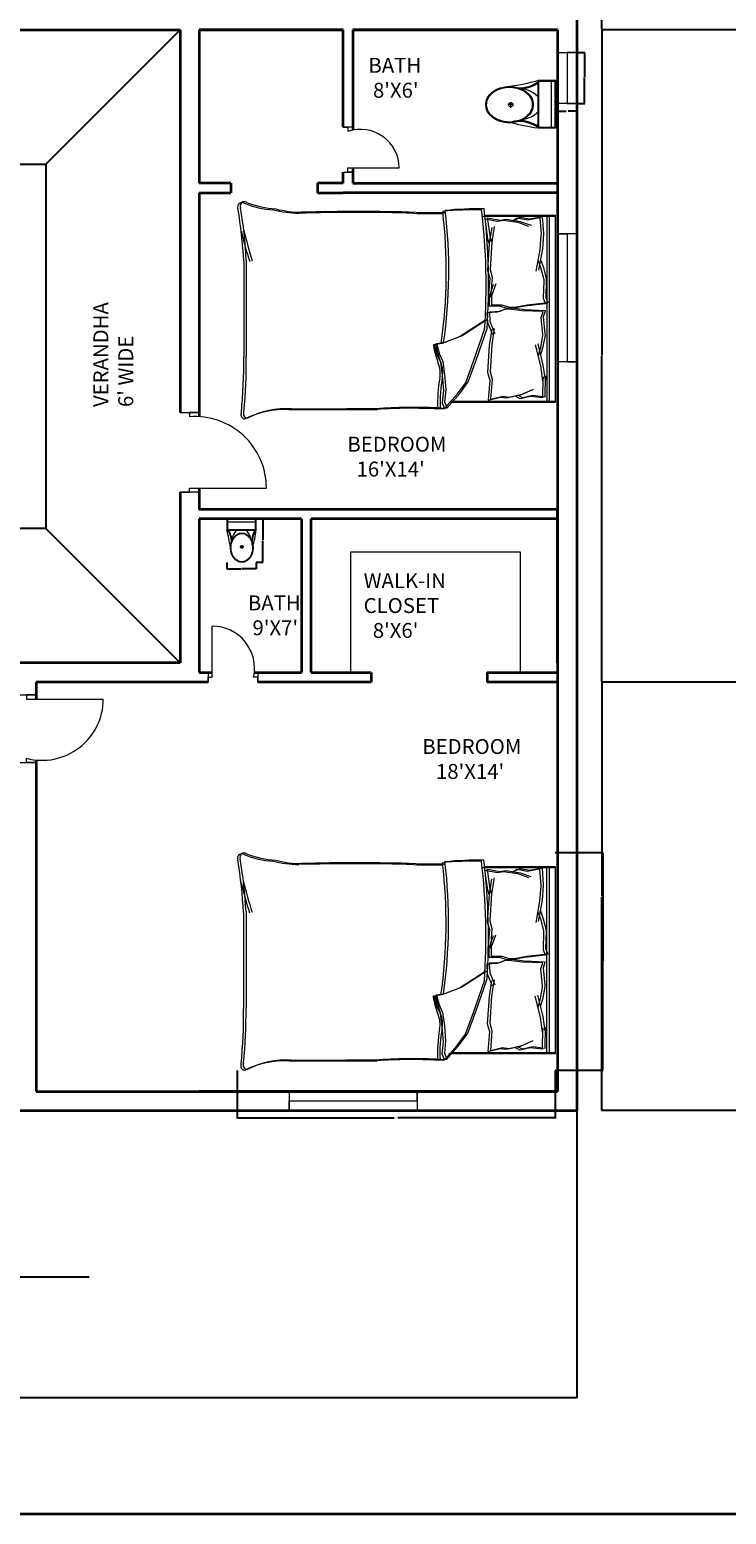
# Model space of a CAD drawing. Units: inches. Extents: x 2185 to 4426, y 1138 to 3073.
# Tile 4 of 14: x 2834 to 3160, y 1138 to 1834. Entities that reach past the tile are written whole.
import ezdxf

# ---------------------------------------------------------------- set-up
doc = ezdxf.new("R2010")
doc.units = ezdxf.units.IN
for name, color, linetype, lineweight in [('A-ANNO-DIMS', 2, 'Continuous', 18), ('A-ANNO-TITL', 7, 'Continuous', 25), ('A-ANNO-TTLB', 7, 'Continuous', 35), ('A-AREA-IDEN', 7, 'Continuous', 18), ('A-DOOR', 3, 'Continuous', 18), ('A-FLOR-CASE', 32, 'Continuous', 18), ('A-FLOR-EDGE', 7, 'Continuous', 25), ('A-FLOR-FIXT', 9, 'Continuous', 18), ('A-FURN', 8, 'Continuous', 18), ('A-GLAZ', 4, 'Continuous', 18), ('A-WALL', 7, 'Continuous', 35)]:
    doc.layers.add(name, color=color, linetype=linetype, lineweight=lineweight)
doc.styles.get("Standard").update_dxf_attribs({"font": 'arial.ttf'})
doc.dimstyles.get("Standard").update_dxf_attribs({"dimtxt": 0.18, "dimasz": 0.18, "dimexe": 0.18, "dimexo": 0.0625, "dimgap": 0.09, "dimtad": 0, "dimtih": 1, "dimtoh": 1, "dimdec": 4, "dimzin": 0, "dimdsep": 46, "dimtxsty": 'Standard', "dimcen": 0.09, "dimadec": 0, "dimazin": 0, "dimtfac": 1, "dimtdec": 4, "dimtofl": 0, "dimtmove": 0, "dimatfit": 3, "dimfxl": 1, "dimtolj": 1, "dimtzin": 0, "dimarcsym": 0})

# ---------------------------------------------------------------- blocks, each defined once
blk = doc.blocks.new('A$C31115884')
for p, q in [((283, 498), (223, 498)), ((258, 466), (258, 523)), ((0, 200), (0, 0)), ((520, 200), (0, 200)), ((10, 190), (10, 10)), ((510, 190), (10, 190)), ((510, 10), (510, 190)), ((520, 0), (520, 200)), ((510, 54), (0, 54)), ((10, 10), (510, 10)), ((0, 0), (520, 0))]:
    blk.add_line(p, q)
blk.add_circle((256, 496), 23.6)
for centre, radius, start, end in [((2778, -205), 2807, 165.4549, 171.7133), ((3237, 905), 2807, 188.2867, 194.5451), ((-295, 403), 365, 324.2091, 9.3499), ((-295, 403), 375, 324.2091, 9.3499), ((384, 406), 293, 190.2774, 224.1564), ((139, 406), 293, 315.8436, 2.6563), ((806, 403), 375, 179.2036, 215.7909), ((806, 403), 365, 170.6501, 215.7909)]:
    blk.add_arc(centre, radius, start, end)
blk.add_ellipse((256, 510), major_axis=(0, -261), ratio=0.772727)
blk.add_open_spline([(256, 259), (263, 259), (270, 260), (288, 262), (299, 265), (320, 273), (330, 278), (350, 291), (360, 299), (378, 316), (386, 326), (402, 347), (409, 358), (421, 383), (427, 395), (436, 422), (440, 436), (445, 465), (447, 480), (448, 509), (448, 524), (445, 553), (443, 568), (436, 596), (432, 610), (422, 636), (416, 649), (402, 672), (395, 683), (379, 703), (370, 712), (351, 728), (341, 735), (321, 746), (310, 751), (289, 757), (278, 759), (256, 761), (245, 761), (223, 757), (212, 754), (191, 746), (181, 741), (161, 728), (151, 720), (133, 703), (125, 693), (110, 672), (103, 660), (90, 636), (85, 623), (76, 596), (72, 582), (67, 553), (66, 538), (64, 509), (65, 494), (68, 465), (70, 450), (77, 422), (81, 408), (91, 382), (97, 370), (111, 346), (118, 335), (135, 316), (144, 307), (162, 291), (172, 284), (193, 273), (203, 269), (225, 262), (236, 260), (250, 259), (253, 259), (256, 259)], degree=3, knots=[0, 0, 0, 0, 0.110105, 0.110105, 0.285049, 0.285049, 0.459994, 0.459994, 0.634938, 0.634938, 0.809882, 0.809882, 0.984827, 0.984827, 1.159771, 1.159771, 1.334715, 1.334715, 1.50966, 1.50966, 1.684604, 1.684604, 1.859549, 1.859549, 2.034493, 2.034493, 2.209437, 2.209437, 2.384382, 2.384382, 2.559326, 2.559326, 2.73427, 2.73427, 2.909215, 2.909215, 3.084159, 3.084159, 3.259103, 3.259103, 3.434048, 3.434048, 3.608992, 3.608992, 3.783936, 3.783936, 3.958881, 3.958881, 4.133825, 4.133825, 4.30877, 4.30877, 4.483714, 4.483714, 4.658658, 4.658658, 4.833603, 4.833603, 5.008547, 5.008547, 5.183491, 5.183491, 5.358436, 5.358436, 5.53338, 5.53338, 5.708324, 5.708324, 5.883269, 5.883269, 6.058213, 6.058213, 6.233158, 6.233158, 6.283185, 6.283185, 6.283185, 6.283185])
blk = doc.blocks.new('BED-DOUBLE')
for p, q in [((0, 93.75), (0, 94.16)), ((0, 94.16), (1.36, 94.16)), ((0, 93.75), (48.66, 93.75)), ((0, 6.35), (0, 93.75)), ((1.17, 94.16), (49.83, 94.16)), ((2.8, 6.35), (2.8, 93.75)), ((3.97, 6.77), (3.97, 94.16)), ((4.68, 91.64), (4.5, 81.76)), ((4.68, 91.64), (10.55, 90.94)), ((5.85, 92.05), (5.67, 82.18)), ((5.85, 92.05), (11.72, 91.36)), ((10.55, 90.94), (15.25, 92.03)), ((16.27, 90.59), (11.37, 88.43)), ((11.72, 91.36), (16.42, 92.45)), ((21.63, 91.64), (15.1, 90.17)), ((15.25, 92.03), (17.16, 91.09)), ((22.8, 92.05), (16.27, 90.59)), ((16.42, 92.45), (18.33, 91.51)), ((24.57, 91.29), (21.63, 91.64)), ((25.74, 91.71), (22.8, 92.05)), ((30.31, 92.71), (24.57, 91.29)), ((31.48, 93.13), (25.74, 91.71)), ((29.57, 83.32), (30.31, 92.71)), ((30.74, 83.74), (31.48, 93.13)), ((50.74, 96.68), (44.79, 89.9)), ((51.91, 97.09), (45.96, 90.32)), ((53.93, 96.82), (50.74, 96.68, 7.08)), ((51.87, 93.87), (50.74, 96.68)), ((51.3, 88.2), (51.87, 93.87)), ((55.1, 97.24), (51.91, 97.09, 7.08)), ((53.04, 94.28), (51.91, 97.09)), ((52.47, 88.62), (53.04, 94.28)), ((4.5, 81.76), (4.65, 83.59)), ((4.65, 83.59), (5.61, 76.65)), ((5.67, 82.18), (5.82, 84.01)), ((5.82, 84.01), (6.78, 77.06)), ((15.1, 90.17), (10.2, 88.01)), ((31.76, 80.16), (30.74, 83.74)), ((40.83, 84.52), (37.15, 74.32)), ((42, 84.94), (38.32, 74.74)), ((44.79, 89.9), (40.83, 84.52)), ((45.96, 90.32), (42, 84.94)), ((51.87, 81.12), (51.3, 88.2)), ((53.04, 81.54), (52.47, 88.62)), ((5.61, 76.65), (8.09, 66.74)), ((6.78, 77.06), (9.26, 67.15)), ((30.59, 79.74), (29.57, 83.32)), ((29.8, 66.92), (30.59, 79.74)), ((30.97, 67.34), (31.76, 80.16)), ((52.72, 74.89), (51.87, 81.12)), ((53.89, 75.31), (53.04, 81.54)), ((6.72, 71.68), (5.63, 67.91)), ((7.89, 72.1), (6.8, 68.32)), ((37.15, 74.32), (31.79, 59.08)), ((38.32, 74.74), (32.96, 59.49)), ((54.42, 71.21), (52.72, 74.89)), ((55.59, 71.63), (53.89, 75.31)), ((55.55, 66.68), (54.42, 71.21)), ((56.72, 67.09), (55.59, 71.63)), ((144.91, 27.55), (144.91, 72.56)), ((146.08, 27.96), (146.08, 72.97)), ((5.63, 67.91), (4.64, 62.55)), ((6.8, 68.32), (5.81, 62.97)), ((5.81, 62.97), (5.85, 62.38)), ((28.58, 59.55), (29.8, 66.92)), ((29.75, 59.97), (30.97, 67.34)), ((31.79, 55.33), (43.66, 63)), ((32.96, 55.75), (44.83, 63.41)), ((43.66, 63), (51.87, 66.11)), ((44.83, 63.41), (53.04, 66.53)), ((51.87, 66.11), (55.55, 66.68)), ((53.04, 66.53), (56.72, 67.09)), ((4.64, 62.55), (4.68, 61.96)), ((4.68, 61.96), (5.45, 53.86)), ((5.85, 62.38), (6.62, 54.28)), ((30.61, 56.23), (28.26, 61.85)), ((31.78, 56.65), (29.43, 62.26)), ((30.89, 51.75), (30.61, 56.23)), ((32.06, 52.16), (31.78, 56.65)), ((5.45, 53.86), (4.56, 51.16)), ((4.56, 51.16), (14.39, 50.71)), ((4.59, 47.93), (14.37, 48.99)), ((6.62, 54.28), (5.73, 51.58)), ((5.73, 51.58), (15.56, 51.13)), ((13.2, 48.57), (19.02, 49.63)), ((14.37, 48.99), (20.19, 50.05)), ((14.39, 50.71), (20.26, 50.02)), ((15.56, 51.13), (21.43, 50.44)), ((19.02, 49.63), (21.4, 49.63)), ((20.19, 50.05), (22.57, 50.05)), ((20.26, 50.02), (22.63, 50.17)), ((21.4, 49.63), (24.84, 48.57)), ((21.43, 50.44), (23.8, 50.59)), ((22.57, 50.05), (26.01, 48.99)), ((22.63, 50.17), (26, 51.44)), ((23.8, 50.59), (27.17, 51.86)), ((26, 51.44), (30.89, 51.75)), ((26.01, 48.99), (30.91, 48.99)), ((27.17, 51.86), (32.06, 52.16)), ((30.91, 48.99), (30.91, 44.49)), ((3.42, 47.51), (13.2, 48.57)), ((4.48, 44.87), (3.42, 47.51)), ((4.21, 36.74), (4.48, 44.87)), ((5.65, 45.29), (4.59, 47.93)), ((5.38, 37.16), (5.65, 45.29)), ((24.84, 48.57), (29.74, 48.57)), ((29.74, 44.08), (27.75, 38.33)), ((30.91, 44.49), (28.91, 38.74)), ((29.57, 35.45), (30.31, 44.83)), ((29.74, 48.57), (29.74, 44.08)), ((30.74, 35.86), (31.48, 45.25)), ((4.21, 36.15), (4.21, 36.74)), ((5.54, 30.86), (4.21, 36.15)), ((5.38, 36.57), (5.38, 37.16)), ((6.7, 31.28), (5.38, 36.57)), ((30.59, 31.86), (29.57, 35.45)), ((31.76, 32.28), (30.74, 35.86)), ((6.86, 27.16), (5.54, 30.86)), ((6.06, 22.14), (7.92, 32.19)), ((8.03, 27.58), (6.7, 31.28)), ((7.23, 22.56), (9.08, 32.6)), ((29.8, 19.04), (30.59, 31.86)), ((30.97, 19.46), (31.76, 32.28)), ((5.54, 15.15), (6.06, 22.14)), ((6.7, 15.57), (7.23, 22.56)), ((5.5, 14.96), (5.54, 15.15)), ((6.1, 7.13), (5.5, 14.96)), ((6.67, 15.37), (6.7, 15.57)), ((7.27, 7.55), (6.67, 15.37)), ((28.58, 11.67), (29.8, 19.04)), ((29.75, 12.09), (30.97, 19.46)), ((29.8, 19.04), (30.39, 16.97)), ((30.39, 16.97), (31.71, 7.65)), ((30.97, 19.46), (31.56, 17.39)), ((31.56, 17.39), (32.88, 8.07)), ((6.06, 7.12), (11.88, 8.18)), ((7.23, 7.54), (13.05, 8.6)), ((16.38, 9.24), (11.35, 11.09)), ((11.88, 8.18), (16.64, 7.39)), ((17.55, 9.65), (12.52, 11.5)), ((13.05, 8.6), (17.81, 7.8)), ((22.99, 8.18), (16.38, 9.24)), ((16.64, 7.39), (18.49, 8.44)), ((24.16, 8.6), (17.55, 9.65)), ((17.81, 7.8), (19.66, 8.86)), ((25.89, 8.71), (22.99, 8.18)), ((27.06, 9.13), (24.16, 8.6)), ((31.71, 7.65), (25.89, 8.71)), ((32.88, 8.07), (27.06, 9.13)), ((1.17, 6.77), (0, 6.77)), ((33.12, 6.35), (0, 6.35)), ((34.29, 6.77), (1.17, 6.77))]:
    blk.add_line(p, q)
for centre, radius, start, end in [((125.19, -8244.52), 8342.06, 90.002168, 90.286887), ((125.57, 139.26), 42.18, 267.47136, 296.46809), ((126.74, 139.68), 42.18, 267.47136, 296.46809), ((144.23, 99.5), 2.02, 332.65876, 86.02002), ((388.18, 75.25), 243.28, 174.4998, 180.63509), ((145.4, 99.91), 2.02, 332.65876, 86.02002), ((389.35, 75.67), 243.28, 174.4998, 180.63509), ((-12.17, 93.86), 66.17, 349.87628, 2.56571), ((66.41, 333.3), 236.81, 266.97912, 273.83645), ((-11, 94.28), 66.17, 349.87628, 2.56571), ((67.58, 333.72), 236.81, 266.97912, 273.83645), ((124.02, -8244.93), 8342.06, 90.002168, 90.286887), ((64.12, 79.99), 11.38, 168.6608, 203.73842), ((65.29, 80.41), 11.38, 168.6608, 203.73842), ((2.71, 56.97), 54.23, 10.66171, 19.88058), ((3.88, 57.39), 54.23, 10.66171, 19.88058), ((285.85, 32.47), 235.93, 171.78449, 186.90062), ((287.02, 32.89), 235.93, 171.78449, 186.90062), ((55.66, 66.99), 0.337, 250.24637, 1.13765), ((56.83, 67.41), 0.337, 250.24637, 1.13765), ((332.91, 39.06), 301.67, 176.08655, 186.78213), ((334.08, 39.47), 301.67, 176.08655, 186.78213), ((-42.19, -31.08), 194.68, 13.38322, 17.70533), ((368.43, 39.6), 222.65, 182.99578, 189.40907), ((-43.36, -31.49), 194.68, 13.38322, 17.70533), ((367.26, 39.18), 222.65, 182.99578, 189.40907), ((36.75, 155.73), 152.34, 268.72178, 275.60397), ((37.92, 156.15), 152.34, 268.72178, 275.60397), ((57.01, -305.95), 311.07, 88.4762, 91.00819), ((58.18, -305.53), 311.07, 88.4762, 91.00819), ((92.56, 886.57), 881.98, 268.22771, 271.71854), ((93.72, 886.99), 881.98, 268.22771, 271.71854), ((117.98, -49.19), 54.19, 76.06484, 88.91125), ((119.15, -48.77), 54.19, 76.06484, 88.91125), ((128.51, -39.61), 43.09, 67.97508, 86.652), ((129.68, -39.19), 43.09, 67.97508, 86.652), ((145.78, 1.99), 1.99, 236.17358, 23.47814), ((146.95, 2.41), 1.99, 236.17358, 23.47814)]:
    blk.add_arc(centre, radius, start, end)
blk = doc.blocks.new('DOOR-SGL-24-BATH-S')
for p, q in [((2, 2.25), (2, 26.25)), ((0, 4.5), (0, 0)), ((0, 0), (0, 2.25)), ((0, 2.25), (0, 2.25)), ((0, 2.25), (2, 2.25)), ((23.36, 2.25), (21.36, 2.25)), ((23.36, 4.5), (23.36, 4.5)), ((23.36, 4.5), (23.36, 0)), ((23.36, 0), (23.36, 2.25))]:
    blk.add_line(p, q)
blk.add_arc((2, 6.44), 19.81, 347.78651, 90)
blk = doc.blocks.new('DOOR-SGL-36-BED-SE')
for p, q in [((0, 37.45), (9, 37.45)), ((9, 37.45), (4.5, 37.45)), ((4.5, 37.45), (4.5, 35.45)), ((9, 0), (0, 0)), ((0, 0), (4.5, 0)), ((4.5, 0), (4.5, 2)), ((4.5, 2), (40.5, 2))]:
    blk.add_line(p, q)
blk.add_arc((6.96, 2), 33.54, 0, 94.21362)
blk = doc.blocks.new('DOOR-SGL-24-BATH-E')
for p, q in [((4.5, 21.05), (0, 21.05)), ((0, 21.05), (2.25, 21.05)), ((2.25, 21.05), (2.25, 19.05)), ((0, 0), (4.5, 0)), ((2.25, 0), (2.25, 2)), ((2.25, 2), (26.25, 2)), ((4.5, 0), (2.25, 0))]:
    blk.add_line(p, q)
blk.add_arc((8.19, 2), 18.06, 0, 109.21567)
blk = doc.blocks.new('DOOR-SGL-36-BED-S')
for p, q in [((0, 31.73), (9, 31.73)), ((9, 31.73), (4.5, 31.73)), ((4.5, 31.73), (4.5, 31.73)), ((4.5, 31.73), (4.5, 29.73)), ((4.5, 29.73), (40.5, 29.73)), ((0, 0), (9, 0)), ((4.5, 0), (4.5, 2)), ((9, 0), (4.5, 0))]:
    blk.add_line(p, q)
blk.add_arc((11.82, 29.73), 28.68, 255.21093, 0)
blk = doc.blocks.new('WIN-PLAN-24IN-03')
for p, q in [((0, 24), (9, 24)), ((9, 24), (4.5, 24)), ((4.5, 24), (4.5, 0)), ((9, 0), (0, 0)), ((4.5, 0), (9, 0))]:
    blk.add_line(p, q)
blk = doc.blocks.new('WIN-PLAN-60IN-01')
for p, q in [((0, 9), (0, 0)), ((60, 4.5), (60, 9)), ((60, 9), (60, 0)), ((0, 0), (0, 4.5)), ((0, 4.5), (0, 4.5)), ((0, 4.5), (60, 4.5))]:
    blk.add_line(p, q)
blk = doc.blocks.new('WARDROBE-U')
for p, q in [((0, 0), (0, 56.6)), ((0, 56.6), (79.32, 56.6)), ((79.32, 56.6), (79.32, 0))]:
    blk.add_line(p, q)
blk = doc.blocks.new('*D46')
at = {"layer": 'A-ANNO-DIMS', "color": 0, "lineweight": -2, "transparency": 16777216}
for p, q in [((2930.76, 1346.2), (2930.76, 1323.71)), ((3079.88, 1346.2), (3079.88, 1323.71)), ((2930.94, 1323.89), (3004.43, 1323.89)), ((3079.7, 1323.89), (3006.21, 1323.89))]:
    blk.add_line(p, q, dxfattribs=at)
at = {"layer": 'A-ANNO-DIMS', "color": 0, "transparency": 16777216}
for points in [[(2930.94, 1323.92), (2930.94, 1323.86), (2930.76, 1323.89)], [(3079.7, 1323.92), (3079.7, 1323.86), (3079.88, 1323.89)]]:
    blk.add_solid(points, dxfattribs=at)
at = {"layer": 'Defpoints', "color": 0, "transparency": 16777216}
for p in [(2930.76, 1346.26), (3079.88, 1346.26), (2930.76, 1323.89)]:
    blk.add_point(p, dxfattribs=at)
at = {"layer": 'A-ANNO-DIMS', "color": 0, "transparency": 16777216, "insert": (3005.32, 1323.89), "char_height": 0.18, "attachment_point": 5}
blk.add_mtext('\\A1;BED 149 TYP.', dxfattribs=at)
blk = doc.blocks.new('*D47')
at = {"layer": 'A-ANNO-DIMS', "color": 0, "lineweight": -2, "transparency": 16777216}
for p, q in [((3079.94, 1448.35), (3102.43, 1448.35)), ((3102.25, 1448.17), (3102.25, 1397.49)), ((3102.25, 1346.44), (3102.25, 1397.12)), ((3079.94, 1346.26), (3102.43, 1346.26))]:
    blk.add_line(p, q, dxfattribs=at)
at = {"layer": 'A-ANNO-DIMS', "color": 0, "transparency": 16777216}
for points in [[(3102.22, 1448.17), (3102.28, 1448.17), (3102.25, 1448.35)], [(3102.22, 1346.44), (3102.28, 1346.44), (3102.25, 1346.26)]]:
    blk.add_solid(points, dxfattribs=at)
at = {"layer": 'Defpoints', "color": 0, "transparency": 16777216}
for p in [(3079.88, 1448.35), (3079.88, 1346.26), (3102.25, 1346.26)]:
    blk.add_point(p, dxfattribs=at)
at = {"layer": 'A-ANNO-DIMS', "color": 0, "transparency": 16777216, "insert": (3102.25, 1397.3), "char_height": 0.18, "attachment_point": 5}
blk.add_mtext('\\A1;102 TYP.', dxfattribs=at)
blk = doc.blocks.new('*D50')
at = {"layer": 'A-ANNO-DIMS', "color": 0, "lineweight": -2, "transparency": 16777216}
for p, q in [((2939.8, 1604.88), (2942.96, 1604.88)), ((2942.78, 1604.7), (2942.78, 1594.9)), ((2942.78, 1584.73), (2942.78, 1594.53)), ((2939.8, 1584.55), (2942.96, 1584.55))]:
    blk.add_line(p, q, dxfattribs=at)
at = {"layer": 'A-ANNO-DIMS', "color": 0, "transparency": 16777216}
for points in [[(2942.75, 1604.7), (2942.81, 1604.7), (2942.78, 1604.88)], [(2942.75, 1584.73), (2942.81, 1584.73), (2942.78, 1584.55)]]:
    blk.add_solid(points, dxfattribs=at)
at = {"layer": 'Defpoints', "color": 0, "transparency": 16777216}
for p in [(2939.73, 1604.88), (2939.73, 1584.55), (2942.78, 1584.55)]:
    blk.add_point(p, dxfattribs=at)
at = {"layer": 'A-ANNO-DIMS', "color": 0, "transparency": 16777216, "insert": (2942.78, 1594.71), "char_height": 0.18, "attachment_point": 5}
blk.add_mtext('\\A1;WC 20', dxfattribs=at)
blk = doc.blocks.new('*D51')
at = {"layer": 'A-ANNO-DIMS', "color": 0, "lineweight": -2, "transparency": 16777216}
for p, q in [((2926.02, 1584.49), (2926.02, 1581.32)), ((2926.2, 1581.5), (2932.66, 1581.5)), ((2939.55, 1581.5), (2933.08, 1581.5)), ((2939.73, 1584.49), (2939.73, 1581.32))]:
    blk.add_line(p, q, dxfattribs=at)
at = {"layer": 'A-ANNO-DIMS', "color": 0, "transparency": 16777216}
for points in [[(2926.2, 1581.53), (2926.2, 1581.47), (2926.02, 1581.5)], [(2939.55, 1581.53), (2939.55, 1581.47), (2939.73, 1581.5)]]:
    blk.add_solid(points, dxfattribs=at)
at = {"layer": 'Defpoints', "color": 0, "transparency": 16777216}
for p in [(2926.02, 1584.55), (2926.02, 1581.5), (2939.73, 1584.55)]:
    blk.add_point(p, dxfattribs=at)
at = {"layer": 'A-ANNO-DIMS', "color": 0, "transparency": 16777216, "insert": (2932.87, 1581.5), "char_height": 0.18, "attachment_point": 5}
blk.add_mtext('\\A1;14', dxfattribs=at)
blk = doc.blocks.new('*D94')
at = {"layer": 'A-ANNO-DIMS', "color": 0, "lineweight": -2, "transparency": 16777216}
for p, q in [((3090.08, 1823.71), (3093.8, 1823.71)), ((3093.62, 1823.53), (3093.62, 1811.9)), ((3093.62, 1799.89), (3093.62, 1811.53)), ((3090.08, 1799.71), (3093.8, 1799.71))]:
    blk.add_line(p, q, dxfattribs=at)
at = {"layer": 'A-ANNO-DIMS', "color": 0, "transparency": 16777216}
for points in [[(3093.59, 1823.53), (3093.65, 1823.53), (3093.62, 1823.71)], [(3093.59, 1799.89), (3093.65, 1799.89), (3093.62, 1799.71)]]:
    blk.add_solid(points, dxfattribs=at)
at = {"layer": 'Defpoints', "color": 0, "transparency": 16777216}
for p in [(3090.02, 1823.71), (3093.62, 1823.71), (3090.02, 1799.71)]:
    blk.add_point(p, dxfattribs=at)
at = {"layer": 'A-ANNO-DIMS', "color": 0, "transparency": 16777216, "insert": (3093.62, 1811.71), "char_height": 0.18, "attachment_point": 5}
blk.add_mtext('\\A1;WINDOW 24 TYP.', dxfattribs=at)
blk = doc.blocks.new('*D95')
at = {"layer": 'A-ANNO-DIMS', "color": 0, "lineweight": -2, "transparency": 16777216}
for p, q in [((3081.02, 1799.65), (3081.02, 1795.93)), ((3090.02, 1799.65), (3090.02, 1795.93)), ((3081.2, 1796.11), (3085.06, 1796.11)), ((3089.84, 1796.11), (3085.98, 1796.11))]:
    blk.add_line(p, q, dxfattribs=at)
at = {"layer": 'A-ANNO-DIMS', "color": 0, "transparency": 16777216}
for points in [[(3081.2, 1796.14), (3081.2, 1796.08), (3081.02, 1796.11)], [(3089.84, 1796.14), (3089.84, 1796.08), (3090.02, 1796.11)]]:
    blk.add_solid(points, dxfattribs=at)
at = {"layer": 'Defpoints', "color": 0, "transparency": 16777216}
for p in [(3081.02, 1799.71), (3090.02, 1799.71), (3090.02, 1796.11)]:
    blk.add_point(p, dxfattribs=at)
at = {"layer": 'A-ANNO-DIMS', "color": 0, "transparency": 16777216, "insert": (3085.52, 1796.11), "char_height": 0.18, "attachment_point": 5}
blk.add_mtext('\\A1;9 TYP.', dxfattribs=at)
blk = doc.blocks.new('*D138')
at = {"layer": 'A-ANNO-DIMS', "color": 0, "lineweight": -2, "transparency": 16777216}
for p, q in [((2368.52, 1327.31), (2368.52, 1192.47)), ((3090.02, 1327.31), (3090.02, 1192.47)), ((2368.7, 1192.65), (2728.88, 1192.65)), ((3089.84, 1192.65), (2729.66, 1192.65))]:
    blk.add_line(p, q, dxfattribs=at)
at = {"layer": 'A-ANNO-DIMS', "color": 0, "transparency": 16777216}
for points in [[(2368.7, 1192.68), (2368.7, 1192.62), (2368.52, 1192.65)], [(3089.84, 1192.68), (3089.84, 1192.62), (3090.02, 1192.65)]]:
    blk.add_solid(points, dxfattribs=at)
at = {"layer": 'Defpoints', "color": 0, "transparency": 16777216}
for p in [(2368.52, 1327.38), (3090.02, 1327.38), (3090.02, 1192.65)]:
    blk.add_point(p, dxfattribs=at)
at = {"layer": 'A-ANNO-DIMS', "color": 0, "transparency": 16777216, "insert": (2729.27, 1192.65), "char_height": 0.18, "attachment_point": 5}
blk.add_mtext('\\A1;721.5', dxfattribs=at)
blk = doc.blocks.new('*D150')
at = {"layer": 'A-ANNO-DIMS', "color": 0, "lineweight": -2, "transparency": 16777216}
for p, q in [((3219.79, 1528.38), (3101.64, 1528.38)), ((3101.82, 1528.2), (3101.82, 1428.06)), ((3101.82, 1327.56), (3101.82, 1427.7)), ((3210.79, 1327.38), (3101.64, 1327.38))]:
    blk.add_line(p, q, dxfattribs=at)
at = {"layer": 'A-ANNO-DIMS', "color": 0, "transparency": 16777216}
for points in [[(3101.79, 1528.2), (3101.85, 1528.2), (3101.82, 1528.38)], [(3101.79, 1327.56), (3101.85, 1327.56), (3101.82, 1327.38)]]:
    blk.add_solid(points, dxfattribs=at)
at = {"layer": 'Defpoints', "color": 0, "transparency": 16777216}
for p in [(3101.82, 1528.38), (3219.85, 1528.38), (3210.85, 1327.38)]:
    blk.add_point(p, dxfattribs=at)
at = {"layer": 'A-ANNO-DIMS', "color": 0, "transparency": 16777216, "insert": (3101.82, 1427.88), "char_height": 0.18, "attachment_point": 5}
blk.add_mtext('\\A1;201', dxfattribs=at)
blk = doc.blocks.new('*D151')
at = {"layer": 'A-ANNO-DIMS', "color": 0, "lineweight": -2, "transparency": 16777216}
for p, q in [((3219.79, 1834.38), (3101.64, 1834.38)), ((3101.82, 1834.2), (3101.82, 1681.56)), ((3101.82, 1528.56), (3101.82, 1681.19)), ((3219.79, 1528.38), (3101.64, 1528.38))]:
    blk.add_line(p, q, dxfattribs=at)
at = {"layer": 'A-ANNO-DIMS', "color": 0, "transparency": 16777216}
for points in [[(3101.79, 1834.2), (3101.85, 1834.2), (3101.82, 1834.38)], [(3101.79, 1528.56), (3101.85, 1528.56), (3101.82, 1528.38)]]:
    blk.add_solid(points, dxfattribs=at)
at = {"layer": 'Defpoints', "color": 0, "transparency": 16777216}
for p in [(3101.82, 1834.38), (3219.85, 1834.38), (3219.85, 1528.38)]:
    blk.add_point(p, dxfattribs=at)
at = {"layer": 'A-ANNO-DIMS', "color": 0, "transparency": 16777216, "insert": (3101.82, 1681.38), "char_height": 0.18, "attachment_point": 5}
blk.add_mtext('\\A1;306', dxfattribs=at)
blk = doc.blocks.new('*D152')
at = {"layer": 'A-ANNO-DIMS', "color": 0, "lineweight": -2, "transparency": 16777216}
for p, q in [((3155.01, 1880.56), (3101.64, 1880.56)), ((3101.82, 1880.38), (3101.82, 1857.65)), ((3101.82, 1834.56), (3101.82, 1857.29)), ((3219.79, 1834.38), (3101.64, 1834.38))]:
    blk.add_line(p, q, dxfattribs=at)
at = {"layer": 'A-ANNO-DIMS', "color": 0, "transparency": 16777216}
for points in [[(3101.79, 1880.38), (3101.85, 1880.38), (3101.82, 1880.56)], [(3101.79, 1834.56), (3101.85, 1834.56), (3101.82, 1834.38)]]:
    blk.add_solid(points, dxfattribs=at)
at = {"layer": 'Defpoints', "color": 0, "transparency": 16777216}
for p in [(3101.82, 1880.56), (3155.07, 1880.56), (3219.85, 1834.38)]:
    blk.add_point(p, dxfattribs=at)
at = {"layer": 'A-ANNO-DIMS', "color": 0, "transparency": 16777216, "insert": (3101.82, 1857.47), "char_height": 0.18, "attachment_point": 5}
blk.add_mtext('\\A1;46.19', dxfattribs=at)

msp = doc.modelspace()

# ---------------------------------------------------------------- linework, layer by layer
at = {"layer": 'A-ANNO-TITL'}
msp.add_line((2861.353, 1249.148), (2569.203, 1249.148), dxfattribs=at)
at = {"layer": 'A-ANNO-TTLB'}
msp.add_lwpolyline([(2184.741, 3073.364), (4426.252, 3073.364), (4426.252, 1137.99), (2184.741, 1137.99)], close=True, dxfattribs=at)
at = {"layer": 'A-FLOR-EDGE'}
for p, q in [((2841.019, 1771.377), (2904.019, 1834.377)), ((2841.019, 1771.377), (2841.019, 1771.377)), ((2841.019, 1600.377), (2904.019, 1537.377))]:
    msp.add_line(p, q, dxfattribs=at)
msp.add_lwpolyline([(2569.478, 1771.377), (2841.019, 1771.377), (2841.019, 1600.377), (2569.478, 1600.377)], close=True, dxfattribs=at)
at = {"layer": 'A-WALL'}
for p, q in [((3090.019, 2326.377), (3090.019, 1327.377)), ((2711.156, 1834.377), (2836.519, 1834.377)), ((2836.519, 1834.377), (2904.019, 1834.377)), ((2904.019, 1834.377), (2904.019, 1654.82)), ((2913.019, 1834.377), (2913.019, 1762.377)), ((2980.519, 1834.377), (2913.019, 1834.377)), ((2913.019, 1834.377), (2980.519, 1834.377)), ((2980.519, 1788.614), (2980.519, 1834.377)), ((3081.019, 1834.377), (2985.019, 1834.377)), ((2985.019, 1834.377), (2985.019, 1787.239)), ((3081.019, 1834.377), (2985.019, 1834.377)), ((2985.019, 1834.377), (3081.019, 1834.377)), ((3081.019, 1834.377), (3081.019, 1336.377)), ((2985.019, 1769.563), (2985.019, 1762.377)), ((2927.779, 1762.377), (2913.019, 1762.377)), ((2927.779, 1762.377), (2927.779, 1757.877)), ((2980.519, 1762.377), (2968.538, 1762.377)), ((2968.538, 1762.377), (2968.538, 1757.877)), ((2980.519, 1762.377), (2980.519, 1767.563)), ((2985.019, 1762.377), (3081.019, 1762.377)), ((3081.019, 1762.377), (3081.019, 1757.877)), ((2913.019, 1757.877), (2927.779, 1757.877)), ((2913.019, 1757.877), (2913.019, 1652.849)), ((2968.538, 1757.877), (2980.519, 1757.877)), ((2985.019, 1757.877), (2980.519, 1757.877)), ((3081.019, 1757.877), (2985.019, 1757.877)), ((2904.019, 1617.375), (2904.019, 1537.377)), ((2913.019, 1619.375), (2913.019, 1609.377)), ((3081.019, 1609.377), (2913.019, 1609.377)), ((2985.019, 1609.377), (2961.019, 1609.377)), ((3081.019, 1609.377), (2985.019, 1609.377)), ((3081.019, 1537.377), (3081.019, 1609.377)), ((2961.019, 1604.877), (2913.019, 1604.877)), ((2913.019, 1604.877), (2913.019, 1537.377)), ((2961.019, 1604.877), (2961.019, 1532.877)), ((2965.519, 1532.877), (2965.519, 1604.877)), ((3081.019, 1604.877), (2965.519, 1604.877)), ((3081.019, 1604.877), (2985.019, 1604.877)), ((2904.019, 1537.377), (2746.431, 1537.377)), ((2913.019, 1537.377), (2913.019, 1532.877)), ((2913.019, 1532.877), (2919.165, 1532.877)), ((2938.879, 1532.877), (2961.019, 1532.877)), ((2965.519, 1532.877), (2993.644, 1532.877)), ((2993.644, 1532.877), (2993.644, 1528.377)), ((3048.121, 1532.877), (3048.121, 1528.377)), ((3048.121, 1532.877), (3081.019, 1532.877)), ((2917.165, 1528.377), (2836.519, 1528.377)), ((2836.519, 1528.377), (2836.519, 1520.356)), ((2913.019, 1528.377), (2908.519, 1528.377)), ((2993.644, 1528.377), (2940.526, 1528.377)), ((3081.019, 1528.377), (3048.121, 1528.377)), ((2836.519, 1491.816), (2836.519, 1336.377)), ((2836.519, 1336.377), (3081.019, 1336.377)), ((3081.019, 1336.377), (2913.019, 1336.377)), ((2711.156, 1327.377), (3090.019, 1327.377))]:
    msp.add_line(p, q, dxfattribs=at)

# ---------------------------------------------------------------- block references
at = {"layer": 'A-DOOR'}
for name, p in [('DOOR-SGL-24-BATH-E', (2980.519, 1767.563)), ('DOOR-SGL-36-BED-SE', (2904.019, 1617.375)), ('DOOR-SGL-24-BATH-S', (2917.165, 1528.377)), ('DOOR-SGL-36-BED-S', (2827.519, 1490.627))]:
    msp.add_blockref(name, p, dxfattribs=at)
at = {"layer": 'A-FLOR-CASE'}
msp.add_blockref('WARDROBE-U', (2984.177, 1532.877), dxfattribs=at)
at = {"layer": 'A-FLOR-FIXT'}
for p, xscale, yscale, zscale, rotation in [((3080.294, 1788.274), 0.0427196977339482, 0.0427196977339482, 0.0427196977339482, 89.99999999999999), ((3080.294, 1788.274), 0.0427196977339482, 0.0427196977339482, 0.0427196977339482, 89.99999999999999), ((2939.733, 1604.877), 0.0263803384082921, 0.0263803384082921, 0.0263803384082921, 180)]:
    msp.add_blockref('A$C31115884', p, dxfattribs=dict(at, xscale=xscale, yscale=yscale, zscale=zscale, rotation=rotation))
at = {"layer": 'A-FURN', "rotation": 180}
for p in [(3079.98, 1753.704), (3079.881, 1448.187)]:
    msp.add_blockref('BED-DOUBLE', p, dxfattribs=at)
at = {"layer": 'A-GLAZ'}
for name, p in [('WIN-PLAN-24IN-03', (3081.019, 1799.715)), ('WIN-PLAN-60IN-01', (2955.211, 1327.377))]:
    msp.add_blockref(name, p, dxfattribs=at)
at = {"layer": 'A-GLAZ', "rotation": 270.0000000000013}
msp.add_blockref('WIN-PLAN-60IN-01', (3081.019, 1738.584), dxfattribs=at)

# ---------------------------------------------------------------- texts
at = {"layer": 'A-AREA-IDEN', "char_height": 7, "attachment_point": 1}
for s, width, insert in [("BATH\\P 8'X6'", 126.04692, (2992.368, 1821.144)), ("BEDROOM\\P  16'X14'", 91.51398, (2982.515, 1643.448)), ("WALK-IN\\PCLOSET\\P  8'X6'", 73.37657, (2990.125, 1579.426)), ("BATH\\P 9'X7'", 104.88325, (2935.86, 1569.005)), ("BEDROOM\\P   18'X14'", 229.57153, (3017.633, 1501.631))]:
    msp.add_mtext_dynamic_manual_height_columns(s, width=width, gutter_width=12.5, heights=[0], dxfattribs=dict(at, insert=insert))
at = {"layer": 'A-AREA-IDEN', "insert": (2863.393, 1657.374), "char_height": 7, "attachment_point": 1, "rotation": 90}
msp.add_mtext_dynamic_manual_height_columns("VERANDHA\\P6' WIDE", width=210.80817, gutter_width=12.5, heights=[0], dxfattribs=at)

# ---------------------------------------------------------------- dimensions: what is measured, and where the dimension line sits
at = {"layer": 'A-ANNO-DIMS'}
for base, p1, p2, angle, override, picture, middle in [((3101.824, 1880.563), (3219.849, 1834.377), (3155.074, 1880.563), 90, {"dimdec": 2, "dimlfac": 1, "dimrnd": 0, "dimzin": 0, "dimdsep": 46, "dimlunit": 2}, '*D152', (3101.824, 1857.47)), ((3101.824, 1834.377), (3219.849, 1528.377), (3219.849, 1834.377), 90, {"dimdec": 0, "dimlfac": 1, "dimrnd": 0, "dimzin": 0, "dimdsep": 46, "dimlunit": 2}, '*D151', (3101.824, 1681.377)), ((2926.015, 1581.5), (2939.733, 1584.549), (2926.015, 1584.549), 180, {"dimdec": 0, "dimlfac": 1, "dimrnd": 0, "dimzin": 0, "dimdsep": 46, "dimlunit": 2}, '*D51', (2932.874, 1581.5)), ((3101.824, 1528.377), (3210.849, 1327.377), (3219.849, 1528.377), 90, {"dimdec": 0, "dimlfac": 1, "dimrnd": 0, "dimzin": 0, "dimdsep": 46, "dimlunit": 2}, '*D150', (3101.824, 1427.877))]:
    dim = msp.add_linear_dim(base=base, p1=p1, p2=p2, angle=angle, dimstyle='Standard', override=override, dxfattribs=at)
    dim.commit()
    dim.dimension.update_dxf_attribs({"geometry": picture, "text_midpoint": middle})
for base, p1, p2, angle, text, picture, middle in [((3093.619, 1823.715), (3090.019, 1799.715), (3090.019, 1823.715), 90, 'WINDOW <> TYP.', '*D94', (3093.619, 1811.715)), ((2942.782, 1584.549), (2939.733, 1604.877), (2939.733, 1584.549), 270, 'WC <>', '*D50', (2942.782, 1594.713)), ((3102.249, 1346.262), (3079.881, 1448.345), (3079.881, 1346.262), 270, '<> TYP.', '*D47', (3102.249, 1397.304)), ((2930.756, 1323.893), (3079.881, 1346.262), (2930.756, 1346.262), 180, 'BED <> TYP.', '*D46', (3005.319, 1323.893))]:
    dim = msp.add_linear_dim(base=base, p1=p1, p2=p2, angle=angle, text=text, dimstyle='Standard', override={"dimdec": 0, "dimlfac": 1, "dimrnd": 0, "dimzin": 0, "dimdsep": 46, "dimlunit": 2}, dxfattribs=at)
    dim.commit()
    dim.dimension.update_dxf_attribs({"geometry": picture, "text_midpoint": middle})
dim = msp.add_linear_dim(base=(3090.019, 1796.115), p1=(3081.019, 1799.715), p2=(3090.019, 1799.715), text='<> TYP.', dimstyle='Standard', override={"dimdec": 0, "dimlfac": 1, "dimrnd": 0, "dimzin": 0, "dimdsep": 46, "dimlunit": 2}, dxfattribs=at)
dim.commit()
dim.dimension.update_dxf_attribs({"geometry": '*D95', "text_midpoint": (3085.519, 1796.115)})
dim = msp.add_linear_dim(base=(3090.019, 1192.648), p1=(2368.519, 1327.377), p2=(3090.019, 1327.377), dimstyle='Standard', override={"dimdec": 1, "dimlfac": 1, "dimrnd": 0, "dimzin": 0, "dimdsep": 46, "dimlunit": 2}, dxfattribs=at)
dim.commit()
dim.dimension.update_dxf_attribs({"geometry": '*D138', "text_midpoint": (2729.269, 1192.648)})

doc.saveas('drawing.dxf')
